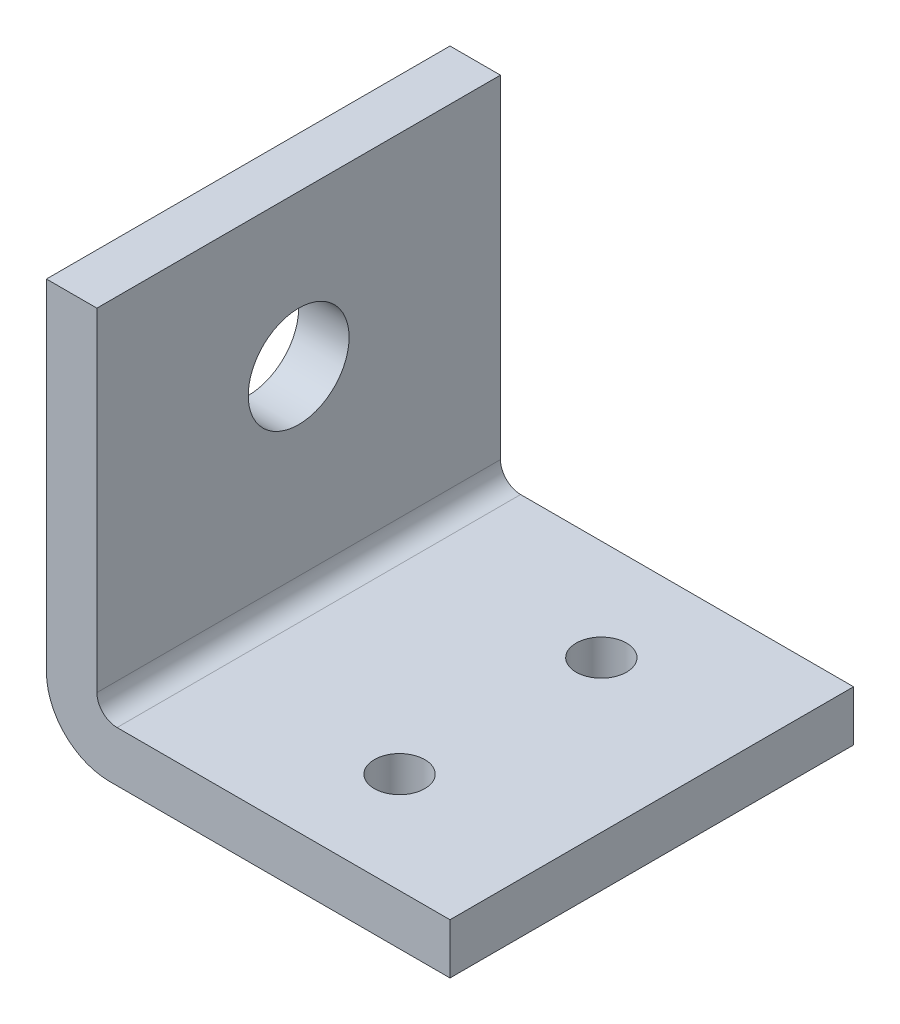
ISO-10303-21;
HEADER;
FILE_DESCRIPTION(('STEP AP214'),'2;1');
FILE_NAME('part.step','',(''),(''),'','','');
FILE_SCHEMA(('AUTOMOTIVE_DESIGN { 1 0 10303 214 1 1 1 1 }'));
ENDSEC;
DATA;
#1=APPLICATION_CONTEXT('core data for automotive mechanical design processes');
#2=APPLICATION_PROTOCOL_DEFINITION('international standard','automotive_design',2000,#1);
#3=PRODUCT_CONTEXT('',#1,'mechanical');
#4=PRODUCT('Part','Part','',(#3));
#5=PRODUCT_RELATED_PRODUCT_CATEGORY('part','',(#4));
#6=PRODUCT_DEFINITION_FORMATION('','',#4);
#7=PRODUCT_DEFINITION_CONTEXT('part definition',#1,'design');
#8=PRODUCT_DEFINITION('design','',#6,#7);
#9=PRODUCT_DEFINITION_SHAPE('','',#8);
#10=(LENGTH_UNIT() NAMED_UNIT(*) SI_UNIT(.MILLI.,.METRE.));
#11=(NAMED_UNIT(*) PLANE_ANGLE_UNIT() SI_UNIT($,.RADIAN.));
#12=(NAMED_UNIT(*) SI_UNIT($,.STERADIAN.) SOLID_ANGLE_UNIT());
#13=UNCERTAINTY_MEASURE_WITH_UNIT(LENGTH_MEASURE(1.E-05),#10,'distance_accuracy_value','');
#14=(GEOMETRIC_REPRESENTATION_CONTEXT(3) GLOBAL_UNCERTAINTY_ASSIGNED_CONTEXT((#13)) GLOBAL_UNIT_ASSIGNED_CONTEXT((#10,
#11,#12)) REPRESENTATION_CONTEXT('',''));
#15=CARTESIAN_POINT('',(0.,0.,0.));
#16=DIRECTION('',(0.,0.,1.));
#17=DIRECTION('',(1.,0.,0.));
#18=AXIS2_PLACEMENT_3D('',#15,#16,#17);
#19=CARTESIAN_POINT('',(0.,40.,20.));
#20=DIRECTION('',(0.,-1.,0.));
#21=DIRECTION('',(0.,0.,-1.));
#22=AXIS2_PLACEMENT_3D('',#19,#20,#21);
#23=PLANE('',#22);
#24=DIRECTION('',(-1.,0.,0.));
#25=VECTOR('',#24,1.);
#26=CARTESIAN_POINT('',(0.,40.,-20.));
#27=LINE('',#26,#25);
#28=CARTESIAN_POINT('',(5.,40.,-20.));
#29=VERTEX_POINT('',#28);
#30=CARTESIAN_POINT('',(0.,40.,-20.));
#31=VERTEX_POINT('',#30);
#32=EDGE_CURVE('E139',#29,#31,#27,.T.);
#33=ORIENTED_EDGE('',*,*,#32,.T.);
#34=DIRECTION('',(0.,0.,-1.));
#35=VECTOR('',#34,1.);
#36=CARTESIAN_POINT('',(0.,40.,20.));
#37=LINE('',#36,#35);
#38=CARTESIAN_POINT('',(0.,40.,20.));
#39=VERTEX_POINT('',#38);
#40=EDGE_CURVE('E11',#39,#31,#37,.T.);
#41=ORIENTED_EDGE('',*,*,#40,.F.);
#42=DIRECTION('',(-1.,0.,0.));
#43=VECTOR('',#42,1.);
#44=CARTESIAN_POINT('',(0.,40.,20.));
#45=LINE('',#44,#43);
#46=CARTESIAN_POINT('',(5.,40.,20.));
#47=VERTEX_POINT('',#46);
#48=EDGE_CURVE('E155',#47,#39,#45,.T.);
#49=ORIENTED_EDGE('',*,*,#48,.F.);
#50=DIRECTION('',(0.,0.,-1.));
#51=VECTOR('',#50,1.);
#52=CARTESIAN_POINT('',(5.,40.,20.));
#53=LINE('',#52,#51);
#54=EDGE_CURVE('E134',#47,#29,#53,.T.);
#55=ORIENTED_EDGE('',*,*,#54,.T.);
#56=EDGE_LOOP('',(#33,#41,#49,#55));
#57=FACE_BOUND('',#56,.T.);
#58=ADVANCED_FACE('F41',(#57),#23,.F.);
#59=CARTESIAN_POINT('',(0.,6.25000000000004,20.));
#60=DIRECTION('',(1.,0.,0.));
#61=DIRECTION('',(0.,0.,-1.));
#62=AXIS2_PLACEMENT_3D('',#59,#60,#61);
#63=PLANE('',#62);
#64=CARTESIAN_POINT('',(0.,25.,0.));
#65=DIRECTION('',(1.,0.,0.));
#66=DIRECTION('',(0.,0.,-1.));
#67=AXIS2_PLACEMENT_3D('',#64,#65,#66);
#68=CIRCLE('',#67,5.);
#69=CARTESIAN_POINT('',(0.,25.,-5.));
#70=VERTEX_POINT('',#69);
#71=EDGE_CURVE('E143',#70,#70,#68,.T.);
#72=ORIENTED_EDGE('',*,*,#71,.T.);
#73=EDGE_LOOP('',(#72));
#74=FACE_BOUND('',#73,.T.);
#75=DIRECTION('',(0.,-1.,0.));
#76=VECTOR('',#75,1.);
#77=CARTESIAN_POINT('',(0.,6.25000000000004,-20.));
#78=LINE('',#77,#76);
#79=CARTESIAN_POINT('',(0.,6.25000000000004,-20.));
#80=VERTEX_POINT('',#79);
#81=EDGE_CURVE('E138',#31,#80,#78,.T.);
#82=ORIENTED_EDGE('',*,*,#81,.T.);
#83=DIRECTION('',(0.,0.,-1.));
#84=VECTOR('',#83,1.);
#85=CARTESIAN_POINT('',(0.,6.25000000000004,20.));
#86=LINE('',#85,#84);
#87=CARTESIAN_POINT('',(0.,6.25000000000004,20.));
#88=VERTEX_POINT('',#87);
#89=EDGE_CURVE('E47',#88,#80,#86,.T.);
#90=ORIENTED_EDGE('',*,*,#89,.F.);
#91=DIRECTION('',(0.,-1.,0.));
#92=VECTOR('',#91,1.);
#93=CARTESIAN_POINT('',(0.,6.25000000000004,20.));
#94=LINE('',#93,#92);
#95=EDGE_CURVE('E99',#39,#88,#94,.T.);
#96=ORIENTED_EDGE('',*,*,#95,.F.);
#97=ORIENTED_EDGE('',*,*,#40,.T.);
#98=EDGE_LOOP('',(#82,#90,#96,#97));
#99=FACE_BOUND('',#98,.T.);
#100=ADVANCED_FACE('F229',(#74,#99),#63,.F.);
#101=CARTESIAN_POINT('',(6.25,6.25,20.));
#102=DIRECTION('',(0.,0.,-1.));
#103=DIRECTION('',(-1.,0.,0.));
#104=AXIS2_PLACEMENT_3D('',#101,#102,#103);
#105=CYLINDRICAL_SURFACE('',#104,6.25);
#106=CARTESIAN_POINT('',(6.25,6.25,-20.));
#107=DIRECTION('',(0.,0.,1.));
#108=DIRECTION('',(-1.,0.,0.));
#109=AXIS2_PLACEMENT_3D('',#106,#107,#108);
#110=CIRCLE('',#109,6.25);
#111=CARTESIAN_POINT('',(6.25000000000005,0.,-20.));
#112=VERTEX_POINT('',#111);
#113=EDGE_CURVE('E141',#80,#112,#110,.T.);
#114=ORIENTED_EDGE('',*,*,#113,.T.);
#115=DIRECTION('',(0.,0.,-1.));
#116=VECTOR('',#115,1.);
#117=CARTESIAN_POINT('',(6.25000000000005,0.,20.));
#118=LINE('',#117,#116);
#119=CARTESIAN_POINT('',(6.25000000000005,0.,20.));
#120=VERTEX_POINT('',#119);
#121=EDGE_CURVE('E157',#120,#112,#118,.T.);
#122=ORIENTED_EDGE('',*,*,#121,.F.);
#123=CARTESIAN_POINT('',(6.25,6.25,20.));
#124=DIRECTION('',(0.,0.,1.));
#125=DIRECTION('',(-1.,0.,0.));
#126=AXIS2_PLACEMENT_3D('',#123,#124,#125);
#127=CIRCLE('',#126,6.25);
#128=EDGE_CURVE('E170',#88,#120,#127,.T.);
#129=ORIENTED_EDGE('',*,*,#128,.F.);
#130=ORIENTED_EDGE('',*,*,#89,.T.);
#131=EDGE_LOOP('',(#114,#122,#129,#130));
#132=FACE_BOUND('',#131,.T.);
#133=ADVANCED_FACE('F164',(#132),#105,.T.);
#134=CARTESIAN_POINT('',(6.25000000000004,0.,20.));
#135=DIRECTION('',(0.,1.,0.));
#136=DIRECTION('',(0.,0.,1.));
#137=AXIS2_PLACEMENT_3D('',#134,#135,#136);
#138=PLANE('',#137);
#139=CARTESIAN_POINT('',(25.,0.,-10.));
#140=DIRECTION('',(0.,1.,0.));
#141=DIRECTION('',(0.,0.,1.));
#142=AXIS2_PLACEMENT_3D('',#139,#140,#141);
#143=CIRCLE('',#142,2.5);
#144=CARTESIAN_POINT('',(25.,0.,-7.5));
#145=VERTEX_POINT('',#144);
#146=EDGE_CURVE('E189',#145,#145,#143,.T.);
#147=ORIENTED_EDGE('',*,*,#146,.T.);
#148=EDGE_LOOP('',(#147));
#149=FACE_BOUND('',#148,.T.);
#150=CARTESIAN_POINT('',(25.,0.,10.));
#151=DIRECTION('',(0.,1.,0.));
#152=DIRECTION('',(0.,0.,1.));
#153=AXIS2_PLACEMENT_3D('',#150,#151,#152);
#154=CIRCLE('',#153,2.5);
#155=CARTESIAN_POINT('',(25.,0.,12.5));
#156=VERTEX_POINT('',#155);
#157=EDGE_CURVE('E191',#156,#156,#154,.T.);
#158=ORIENTED_EDGE('',*,*,#157,.T.);
#159=EDGE_LOOP('',(#158));
#160=FACE_BOUND('',#159,.T.);
#161=DIRECTION('',(1.,0.,0.));
#162=VECTOR('',#161,1.);
#163=CARTESIAN_POINT('',(6.25000000000004,0.,-20.));
#164=LINE('',#163,#162);
#165=CARTESIAN_POINT('',(40.,0.,-20.));
#166=VERTEX_POINT('',#165);
#167=EDGE_CURVE('E144',#112,#166,#164,.T.);
#168=ORIENTED_EDGE('',*,*,#167,.T.);
#169=DIRECTION('',(0.,0.,-1.));
#170=VECTOR('',#169,1.);
#171=CARTESIAN_POINT('',(40.,0.,20.));
#172=LINE('',#171,#170);
#173=CARTESIAN_POINT('',(40.,0.,20.));
#174=VERTEX_POINT('',#173);
#175=EDGE_CURVE('E156',#174,#166,#172,.T.);
#176=ORIENTED_EDGE('',*,*,#175,.F.);
#177=DIRECTION('',(1.,0.,0.));
#178=VECTOR('',#177,1.);
#179=CARTESIAN_POINT('',(6.25000000000004,0.,20.));
#180=LINE('',#179,#178);
#181=EDGE_CURVE('E176',#120,#174,#180,.T.);
#182=ORIENTED_EDGE('',*,*,#181,.F.);
#183=ORIENTED_EDGE('',*,*,#121,.T.);
#184=EDGE_LOOP('',(#168,#176,#182,#183));
#185=FACE_BOUND('',#184,.T.);
#186=ADVANCED_FACE('F175',(#149,#160,#185),#138,.F.);
#187=CARTESIAN_POINT('',(40.,0.,20.));
#188=DIRECTION('',(-1.,0.,0.));
#189=DIRECTION('',(0.,0.,1.));
#190=AXIS2_PLACEMENT_3D('',#187,#188,#189);
#191=PLANE('',#190);
#192=DIRECTION('',(0.,1.,0.));
#193=VECTOR('',#192,1.);
#194=CARTESIAN_POINT('',(40.,0.,-20.));
#195=LINE('',#194,#193);
#196=CARTESIAN_POINT('',(40.,5.,-20.));
#197=VERTEX_POINT('',#196);
#198=EDGE_CURVE('E150',#166,#197,#195,.T.);
#199=ORIENTED_EDGE('',*,*,#198,.T.);
#200=DIRECTION('',(0.,0.,-1.));
#201=VECTOR('',#200,1.);
#202=CARTESIAN_POINT('',(40.,5.,20.));
#203=LINE('',#202,#201);
#204=CARTESIAN_POINT('',(40.,5.,20.));
#205=VERTEX_POINT('',#204);
#206=EDGE_CURVE('E126',#205,#197,#203,.T.);
#207=ORIENTED_EDGE('',*,*,#206,.F.);
#208=DIRECTION('',(0.,1.,0.));
#209=VECTOR('',#208,1.);
#210=CARTESIAN_POINT('',(40.,0.,20.));
#211=LINE('',#210,#209);
#212=EDGE_CURVE('E118',#174,#205,#211,.T.);
#213=ORIENTED_EDGE('',*,*,#212,.F.);
#214=ORIENTED_EDGE('',*,*,#175,.T.);
#215=EDGE_LOOP('',(#199,#207,#213,#214));
#216=FACE_BOUND('',#215,.T.);
#217=ADVANCED_FACE('F180',(#216),#191,.F.);
#218=CARTESIAN_POINT('',(7.00000000000002,5.,20.));
#219=DIRECTION('',(0.,-1.,0.));
#220=DIRECTION('',(0.,0.,-1.));
#221=AXIS2_PLACEMENT_3D('',#218,#219,#220);
#222=PLANE('',#221);
#223=CARTESIAN_POINT('',(25.,5.,-10.));
#224=DIRECTION('',(0.,1.,0.));
#225=DIRECTION('',(0.,0.,1.));
#226=AXIS2_PLACEMENT_3D('',#223,#224,#225);
#227=CIRCLE('',#226,2.5);
#228=CARTESIAN_POINT('',(25.,5.,-7.5));
#229=VERTEX_POINT('',#228);
#230=EDGE_CURVE('E197',#229,#229,#227,.T.);
#231=ORIENTED_EDGE('',*,*,#230,.F.);
#232=EDGE_LOOP('',(#231));
#233=FACE_BOUND('',#232,.T.);
#234=CARTESIAN_POINT('',(25.,5.,10.));
#235=DIRECTION('',(0.,1.,0.));
#236=DIRECTION('',(0.,0.,1.));
#237=AXIS2_PLACEMENT_3D('',#234,#235,#236);
#238=CIRCLE('',#237,2.5);
#239=CARTESIAN_POINT('',(25.,5.,12.5));
#240=VERTEX_POINT('',#239);
#241=EDGE_CURVE('E192',#240,#240,#238,.T.);
#242=ORIENTED_EDGE('',*,*,#241,.F.);
#243=EDGE_LOOP('',(#242));
#244=FACE_BOUND('',#243,.T.);
#245=DIRECTION('',(-1.,0.,0.));
#246=VECTOR('',#245,1.);
#247=CARTESIAN_POINT('',(7.00000000000002,5.,-20.));
#248=LINE('',#247,#246);
#249=CARTESIAN_POINT('',(7.00000000000002,5.,-20.));
#250=VERTEX_POINT('',#249);
#251=EDGE_CURVE('E130',#197,#250,#248,.T.);
#252=ORIENTED_EDGE('',*,*,#251,.T.);
#253=DIRECTION('',(0.,0.,-1.));
#254=VECTOR('',#253,1.);
#255=CARTESIAN_POINT('',(7.00000000000002,5.,20.));
#256=LINE('',#255,#254);
#257=CARTESIAN_POINT('',(7.00000000000002,5.,20.));
#258=VERTEX_POINT('',#257);
#259=EDGE_CURVE('E121',#258,#250,#256,.T.);
#260=ORIENTED_EDGE('',*,*,#259,.F.);
#261=DIRECTION('',(-1.,0.,0.));
#262=VECTOR('',#261,1.);
#263=CARTESIAN_POINT('',(7.00000000000002,5.,20.));
#264=LINE('',#263,#262);
#265=EDGE_CURVE('E114',#205,#258,#264,.T.);
#266=ORIENTED_EDGE('',*,*,#265,.F.);
#267=ORIENTED_EDGE('',*,*,#206,.T.);
#268=EDGE_LOOP('',(#252,#260,#266,#267));
#269=FACE_BOUND('',#268,.T.);
#270=ADVANCED_FACE('F123',(#233,#244,#269),#222,.F.);
#271=CARTESIAN_POINT('',(7.,7.,20.));
#272=DIRECTION('',(0.,0.,-1.));
#273=DIRECTION('',(-1.,0.,0.));
#274=AXIS2_PLACEMENT_3D('',#271,#272,#273);
#275=CYLINDRICAL_SURFACE('',#274,2.);
#276=CARTESIAN_POINT('',(7.,7.,-20.));
#277=DIRECTION('',(0.,0.,-1.));
#278=DIRECTION('',(-1.,0.,0.));
#279=AXIS2_PLACEMENT_3D('',#276,#277,#278);
#280=CIRCLE('',#279,2.);
#281=CARTESIAN_POINT('',(5.,7.,-20.));
#282=VERTEX_POINT('',#281);
#283=EDGE_CURVE('E88',#250,#282,#280,.T.);
#284=ORIENTED_EDGE('',*,*,#283,.T.);
#285=DIRECTION('',(0.,0.,-1.));
#286=VECTOR('',#285,1.);
#287=CARTESIAN_POINT('',(5.,7.,20.));
#288=LINE('',#287,#286);
#289=CARTESIAN_POINT('',(5.,7.,20.));
#290=VERTEX_POINT('',#289);
#291=EDGE_CURVE('E129',#290,#282,#288,.T.);
#292=ORIENTED_EDGE('',*,*,#291,.F.);
#293=CARTESIAN_POINT('',(7.,7.,20.));
#294=DIRECTION('',(0.,0.,-1.));
#295=DIRECTION('',(-1.,0.,0.));
#296=AXIS2_PLACEMENT_3D('',#293,#294,#295);
#297=CIRCLE('',#296,2.);
#298=EDGE_CURVE('E117',#258,#290,#297,.T.);
#299=ORIENTED_EDGE('',*,*,#298,.F.);
#300=ORIENTED_EDGE('',*,*,#259,.T.);
#301=EDGE_LOOP('',(#284,#292,#299,#300));
#302=FACE_BOUND('',#301,.T.);
#303=ADVANCED_FACE('F131',(#302),#275,.F.);
#304=CARTESIAN_POINT('',(5.,7.00000000000002,20.));
#305=DIRECTION('',(-1.,0.,0.));
#306=DIRECTION('',(0.,0.,1.));
#307=AXIS2_PLACEMENT_3D('',#304,#305,#306);
#308=PLANE('',#307);
#309=CARTESIAN_POINT('',(5.,25.,0.));
#310=DIRECTION('',(1.,0.,0.));
#311=DIRECTION('',(0.,0.,-1.));
#312=AXIS2_PLACEMENT_3D('',#309,#310,#311);
#313=CIRCLE('',#312,5.);
#314=CARTESIAN_POINT('',(5.,25.,-5.));
#315=VERTEX_POINT('',#314);
#316=EDGE_CURVE('E183',#315,#315,#313,.T.);
#317=ORIENTED_EDGE('',*,*,#316,.F.);
#318=EDGE_LOOP('',(#317));
#319=FACE_BOUND('',#318,.T.);
#320=DIRECTION('',(0.,1.,0.));
#321=VECTOR('',#320,1.);
#322=CARTESIAN_POINT('',(5.,7.00000000000002,-20.));
#323=LINE('',#322,#321);
#324=EDGE_CURVE('E95',#282,#29,#323,.T.);
#325=ORIENTED_EDGE('',*,*,#324,.T.);
#326=ORIENTED_EDGE('',*,*,#54,.F.);
#327=DIRECTION('',(0.,1.,0.));
#328=VECTOR('',#327,1.);
#329=CARTESIAN_POINT('',(5.,7.00000000000002,20.));
#330=LINE('',#329,#328);
#331=EDGE_CURVE('E60',#290,#47,#330,.T.);
#332=ORIENTED_EDGE('',*,*,#331,.F.);
#333=ORIENTED_EDGE('',*,*,#291,.T.);
#334=EDGE_LOOP('',(#325,#326,#332,#333));
#335=FACE_BOUND('',#334,.T.);
#336=ADVANCED_FACE('F240',(#319,#335),#308,.F.);
#337=CARTESIAN_POINT('',(7.,7.,20.));
#338=DIRECTION('',(0.,0.,-1.));
#339=DIRECTION('',(-1.,0.,0.));
#340=AXIS2_PLACEMENT_3D('',#337,#338,#339);
#341=PLANE('',#340);
#342=ORIENTED_EDGE('',*,*,#48,.T.);
#343=ORIENTED_EDGE('',*,*,#95,.T.);
#344=ORIENTED_EDGE('',*,*,#128,.T.);
#345=ORIENTED_EDGE('',*,*,#181,.T.);
#346=ORIENTED_EDGE('',*,*,#212,.T.);
#347=ORIENTED_EDGE('',*,*,#265,.T.);
#348=ORIENTED_EDGE('',*,*,#298,.T.);
#349=ORIENTED_EDGE('',*,*,#331,.T.);
#350=EDGE_LOOP('',(#342,#343,#344,#345,#346,#347,#348,#349));
#351=FACE_BOUND('',#350,.T.);
#352=ADVANCED_FACE('F113',(#351),#341,.F.);
#353=CARTESIAN_POINT('',(7.,7.,-20.));
#354=DIRECTION('',(0.,0.,-1.));
#355=DIRECTION('',(-1.,0.,0.));
#356=AXIS2_PLACEMENT_3D('',#353,#354,#355);
#357=PLANE('',#356);
#358=ORIENTED_EDGE('',*,*,#32,.F.);
#359=ORIENTED_EDGE('',*,*,#324,.F.);
#360=ORIENTED_EDGE('',*,*,#283,.F.);
#361=ORIENTED_EDGE('',*,*,#251,.F.);
#362=ORIENTED_EDGE('',*,*,#198,.F.);
#363=ORIENTED_EDGE('',*,*,#167,.F.);
#364=ORIENTED_EDGE('',*,*,#113,.F.);
#365=ORIENTED_EDGE('',*,*,#81,.F.);
#366=EDGE_LOOP('',(#358,#359,#360,#361,#362,#363,#364,#365));
#367=FACE_BOUND('',#366,.T.);
#368=ADVANCED_FACE('F171',(#367),#357,.T.);
#369=CARTESIAN_POINT('',(0.,25.,0.));
#370=DIRECTION('',(1.,0.,0.));
#371=DIRECTION('',(0.,0.,-1.));
#372=AXIS2_PLACEMENT_3D('',#369,#370,#371);
#373=CYLINDRICAL_SURFACE('',#372,5.);
#374=ORIENTED_EDGE('',*,*,#71,.F.);
#375=EDGE_LOOP('',(#374));
#376=FACE_BOUND('',#375,.T.);
#377=ORIENTED_EDGE('',*,*,#316,.T.);
#378=EDGE_LOOP('',(#377));
#379=FACE_BOUND('',#378,.T.);
#380=ADVANCED_FACE('F217',(#376,#379),#373,.F.);
#381=CARTESIAN_POINT('',(25.,0.,10.));
#382=DIRECTION('',(0.,1.,0.));
#383=DIRECTION('',(0.,0.,1.));
#384=AXIS2_PLACEMENT_3D('',#381,#382,#383);
#385=CYLINDRICAL_SURFACE('',#384,2.5);
#386=ORIENTED_EDGE('',*,*,#157,.F.);
#387=EDGE_LOOP('',(#386));
#388=FACE_BOUND('',#387,.T.);
#389=ORIENTED_EDGE('',*,*,#241,.T.);
#390=EDGE_LOOP('',(#389));
#391=FACE_BOUND('',#390,.T.);
#392=ADVANCED_FACE('F208',(#388,#391),#385,.F.);
#393=CARTESIAN_POINT('',(25.,0.,-10.));
#394=DIRECTION('',(0.,1.,0.));
#395=DIRECTION('',(0.,0.,1.));
#396=AXIS2_PLACEMENT_3D('',#393,#394,#395);
#397=CYLINDRICAL_SURFACE('',#396,2.5);
#398=ORIENTED_EDGE('',*,*,#146,.F.);
#399=EDGE_LOOP('',(#398));
#400=FACE_BOUND('',#399,.T.);
#401=ORIENTED_EDGE('',*,*,#230,.T.);
#402=EDGE_LOOP('',(#401));
#403=FACE_BOUND('',#402,.T.);
#404=ADVANCED_FACE('F202',(#400,#403),#397,.F.);
#405=CLOSED_SHELL('',(#58,#100,#133,#186,#217,#270,#303,#336,#352,#368,#380,#392,#404));
#406=MANIFOLD_SOLID_BREP('B2',#405);
#407=ADVANCED_BREP_SHAPE_REPRESENTATION('',(#18,#406),#14);
#408=SHAPE_DEFINITION_REPRESENTATION(#9,#407);
ENDSEC;
END-ISO-10303-21;
